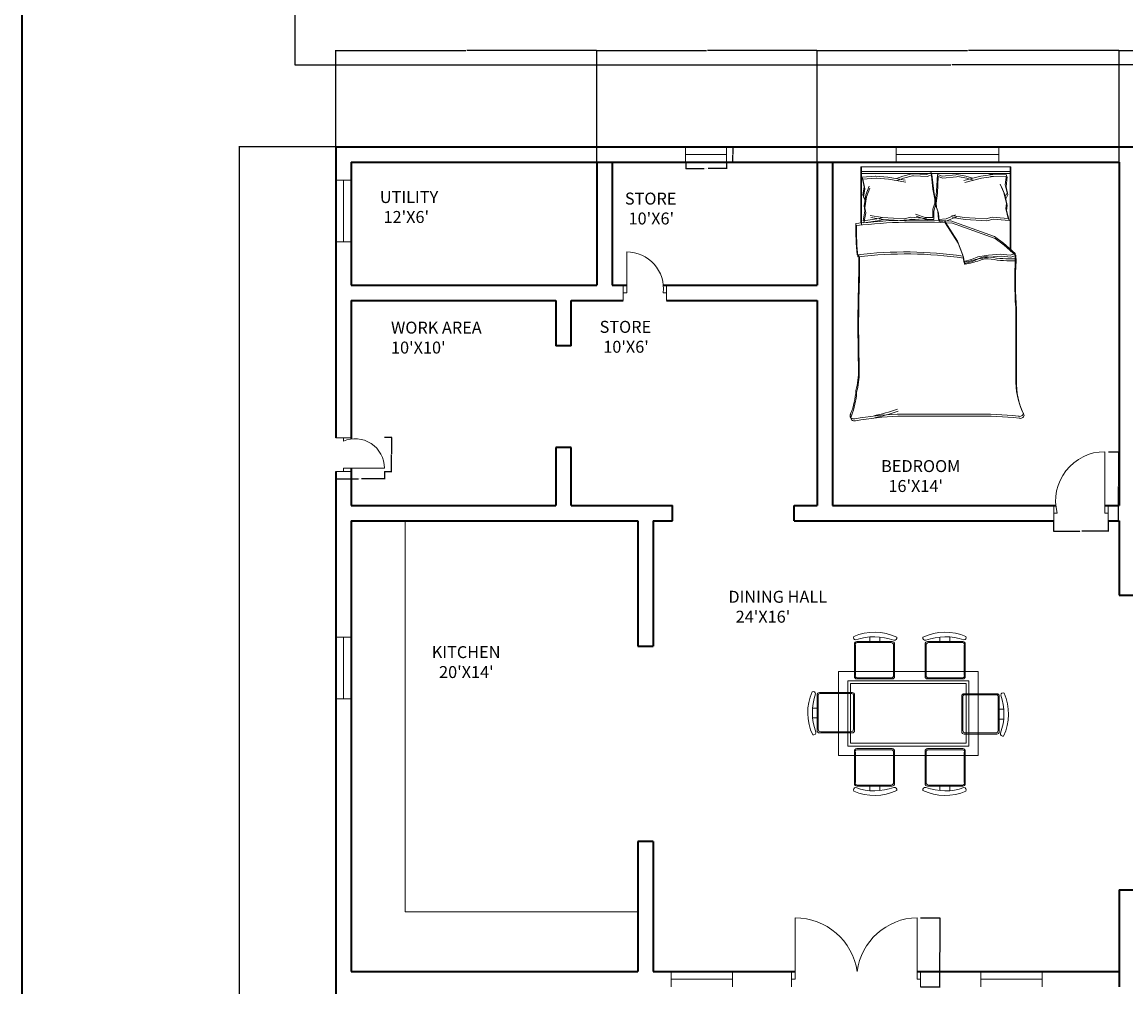
# Model space of a CAD drawing. Units: inches. Extents: x 2185 to 4426, y 1138 to 3073.
# Tile 5 of 14: x 2185 to 2832, y 1834 to 2400. Entities that reach past the tile are written whole.
import ezdxf

# ---------------------------------------------------------------- set-up
doc = ezdxf.new("R2010")
doc.units = ezdxf.units.IN
for name, color, linetype, lineweight in [('A-ANNO-DIMS', 2, 'Continuous', 18), ('A-ANNO-TTLB', 7, 'Continuous', 35), ('A-AREA-IDEN', 7, 'Continuous', 18), ('A-DOOR', 3, 'Continuous', 18), ('A-FLOR-CASE', 32, 'Continuous', 18), ('A-FURN', 8, 'Continuous', 18), ('A-GLAZ', 4, 'Continuous', 18), ('A-WALL', 7, 'Continuous', 35)]:
    doc.layers.add(name, color=color, linetype=linetype, lineweight=lineweight)
doc.styles.get("Standard").update_dxf_attribs({"font": 'arial.ttf'})
doc.dimstyles.get("Standard").update_dxf_attribs({"dimtxt": 0.18, "dimasz": 0.18, "dimexe": 0.18, "dimexo": 0.0625, "dimgap": 0.09, "dimtad": 0, "dimtih": 1, "dimtoh": 1, "dimdec": 4, "dimzin": 0, "dimdsep": 46, "dimtxsty": 'Standard', "dimcen": 0.09, "dimadec": 0, "dimazin": 0, "dimtfac": 1, "dimtdec": 4, "dimtofl": 0, "dimtmove": 0, "dimatfit": 3, "dimfxl": 1, "dimtolj": 1, "dimtzin": 0, "dimarcsym": 0})

# ---------------------------------------------------------------- blocks, each defined once
blk = doc.blocks.new('BED-DOUBLE')
for p, q in [((51.91, 97.09), (45.96, 90.32)), ((55.1, 97.24), (51.91, 97.09, 7.08)), ((53.04, 94.28), (51.91, 97.09)), ((0, 93.75), (0, 94.16)), ((0, 94.16), (1.36, 94.16)), ((0, 93.75), (48.66, 93.75)), ((0, 6.35), (0, 93.75)), ((1.17, 94.16), (49.83, 94.16)), ((2.8, 6.35), (2.8, 93.75)), ((3.97, 6.77), (3.97, 94.16)), ((4.68, 91.64), (4.5, 81.76)), ((4.68, 91.64), (10.55, 90.94)), ((5.85, 92.05), (5.67, 82.18)), ((5.85, 92.05), (11.72, 91.36)), ((10.55, 90.94), (15.25, 92.03)), ((16.27, 90.59), (11.37, 88.43)), ((11.72, 91.36), (16.42, 92.45)), ((21.63, 91.64), (15.1, 90.17)), ((15.25, 92.03), (17.16, 91.09)), ((22.8, 92.05), (16.27, 90.59)), ((16.42, 92.45), (18.33, 91.51)), ((24.57, 91.29), (21.63, 91.64)), ((25.74, 91.71), (22.8, 92.05)), ((30.31, 92.71), (24.57, 91.29)), ((31.48, 93.13), (25.74, 91.71)), ((29.57, 83.32), (30.31, 92.71)), ((30.74, 83.74), (31.48, 93.13)), ((50.74, 96.68), (44.79, 89.9)), ((53.93, 96.82), (50.74, 96.68, 7.08)), ((51.87, 93.87), (50.74, 96.68)), ((51.3, 88.2), (51.87, 93.87)), ((52.47, 88.62), (53.04, 94.28)), ((15.1, 90.17), (10.2, 88.01)), ((40.83, 84.52), (37.15, 74.32)), ((42, 84.94), (38.32, 74.74)), ((44.79, 89.9), (40.83, 84.52)), ((45.96, 90.32), (42, 84.94)), ((51.87, 81.12), (51.3, 88.2)), ((53.04, 81.54), (52.47, 88.62)), ((4.5, 81.76), (4.65, 83.59)), ((4.65, 83.59), (5.61, 76.65)), ((5.67, 82.18), (5.82, 84.01)), ((5.82, 84.01), (6.78, 77.06)), ((30.59, 79.74), (29.57, 83.32)), ((29.8, 66.92), (30.59, 79.74)), ((31.76, 80.16), (30.74, 83.74)), ((30.97, 67.34), (31.76, 80.16)), ((52.72, 74.89), (51.87, 81.12)), ((53.89, 75.31), (53.04, 81.54)), ((5.61, 76.65), (8.09, 66.74)), ((6.72, 71.68), (5.63, 67.91)), ((6.78, 77.06), (9.26, 67.15)), ((7.89, 72.1), (6.8, 68.32)), ((37.15, 74.32), (31.79, 59.08)), ((38.32, 74.74), (32.96, 59.49)), ((54.42, 71.21), (52.72, 74.89)), ((55.59, 71.63), (53.89, 75.31)), ((55.55, 66.68), (54.42, 71.21)), ((56.72, 67.09), (55.59, 71.63)), ((144.91, 27.55), (144.91, 72.56)), ((146.08, 27.96), (146.08, 72.97)), ((5.63, 67.91), (4.64, 62.55)), ((6.8, 68.32), (5.81, 62.97)), ((28.58, 59.55), (29.8, 66.92)), ((29.75, 59.97), (30.97, 67.34)), ((43.66, 63), (51.87, 66.11)), ((44.83, 63.41), (53.04, 66.53)), ((51.87, 66.11), (55.55, 66.68)), ((53.04, 66.53), (56.72, 67.09)), ((4.64, 62.55), (4.68, 61.96)), ((4.68, 61.96), (5.45, 53.86)), ((5.81, 62.97), (5.85, 62.38)), ((5.85, 62.38), (6.62, 54.28)), ((30.61, 56.23), (28.26, 61.85)), ((31.78, 56.65), (29.43, 62.26)), ((31.79, 55.33), (43.66, 63)), ((32.96, 55.75), (44.83, 63.41)), ((5.45, 53.86), (4.56, 51.16)), ((6.62, 54.28), (5.73, 51.58)), ((23.8, 50.59), (27.17, 51.86)), ((26, 51.44), (30.89, 51.75)), ((27.17, 51.86), (32.06, 52.16)), ((30.89, 51.75), (30.61, 56.23)), ((32.06, 52.16), (31.78, 56.65)), ((3.42, 47.51), (13.2, 48.57)), ((4.48, 44.87), (3.42, 47.51)), ((4.56, 51.16), (14.39, 50.71)), ((4.59, 47.93), (14.37, 48.99)), ((5.65, 45.29), (4.59, 47.93)), ((5.38, 37.16), (5.65, 45.29)), ((5.73, 51.58), (15.56, 51.13)), ((13.2, 48.57), (19.02, 49.63)), ((14.37, 48.99), (20.19, 50.05)), ((14.39, 50.71), (20.26, 50.02)), ((15.56, 51.13), (21.43, 50.44)), ((19.02, 49.63), (21.4, 49.63)), ((20.19, 50.05), (22.57, 50.05)), ((20.26, 50.02), (22.63, 50.17)), ((21.4, 49.63), (24.84, 48.57)), ((21.43, 50.44), (23.8, 50.59)), ((22.57, 50.05), (26.01, 48.99)), ((22.63, 50.17), (26, 51.44)), ((24.84, 48.57), (29.74, 48.57)), ((26.01, 48.99), (30.91, 48.99)), ((29.74, 48.57), (29.74, 44.08)), ((30.91, 48.99), (30.91, 44.49)), ((4.21, 36.74), (4.48, 44.87)), ((29.74, 44.08), (27.75, 38.33)), ((30.91, 44.49), (28.91, 38.74)), ((29.57, 35.45), (30.31, 44.83)), ((30.74, 35.86), (31.48, 45.25)), ((4.21, 36.15), (4.21, 36.74)), ((5.54, 30.86), (4.21, 36.15)), ((5.38, 36.57), (5.38, 37.16)), ((6.7, 31.28), (5.38, 36.57)), ((7.23, 22.56), (9.08, 32.6)), ((30.59, 31.86), (29.57, 35.45)), ((31.76, 32.28), (30.74, 35.86)), ((6.86, 27.16), (5.54, 30.86)), ((6.06, 22.14), (7.92, 32.19)), ((8.03, 27.58), (6.7, 31.28)), ((29.8, 19.04), (30.59, 31.86)), ((30.97, 19.46), (31.76, 32.28)), ((5.54, 15.15), (6.06, 22.14)), ((6.7, 15.57), (7.23, 22.56)), ((29.75, 12.09), (30.97, 19.46)), ((30.97, 19.46), (31.56, 17.39)), ((5.5, 14.96), (5.54, 15.15)), ((6.1, 7.13), (5.5, 14.96)), ((6.67, 15.37), (6.7, 15.57)), ((7.27, 7.55), (6.67, 15.37)), ((28.58, 11.67), (29.8, 19.04)), ((29.8, 19.04), (30.39, 16.97)), ((30.39, 16.97), (31.71, 7.65)), ((31.56, 17.39), (32.88, 8.07)), ((1.17, 6.77), (0, 6.77)), ((34.29, 6.77), (1.17, 6.77)), ((6.06, 7.12), (11.88, 8.18)), ((7.23, 7.54), (13.05, 8.6)), ((16.38, 9.24), (11.35, 11.09)), ((11.88, 8.18), (16.64, 7.39)), ((17.55, 9.65), (12.52, 11.5)), ((13.05, 8.6), (17.81, 7.8)), ((22.99, 8.18), (16.38, 9.24)), ((16.64, 7.39), (18.49, 8.44)), ((24.16, 8.6), (17.55, 9.65)), ((17.81, 7.8), (19.66, 8.86)), ((25.89, 8.71), (22.99, 8.18)), ((27.06, 9.13), (24.16, 8.6)), ((31.71, 7.65), (25.89, 8.71)), ((32.88, 8.07), (27.06, 9.13)), ((33.12, 6.35), (0, 6.35))]:
    blk.add_line(p, q)
for centre, radius, start, end in [((66.41, 333.3), 236.81, 266.97912, 273.83645), ((-11, 94.28), 66.17, 349.87628, 2.56571), ((67.58, 333.72), 236.81, 266.97912, 273.83645), ((124.02, -8244.93), 8342.06, 90.002168, 90.286887), ((125.19, -8244.52), 8342.06, 90.002168, 90.286887), ((125.57, 139.26), 42.18, 267.47136, 296.46809), ((126.74, 139.68), 42.18, 267.47136, 296.46809), ((144.23, 99.5), 2.02, 332.65876, 86.02002), ((388.18, 75.25), 243.28, 174.4998, 180.63509), ((145.4, 99.91), 2.02, 332.65876, 86.02002), ((389.35, 75.67), 243.28, 174.4998, 180.63509), ((-12.17, 93.86), 66.17, 349.87628, 2.56571), ((64.12, 79.99), 11.38, 168.6608, 203.73842), ((65.29, 80.41), 11.38, 168.6608, 203.73842), ((2.71, 56.97), 54.23, 10.66171, 19.88058), ((3.88, 57.39), 54.23, 10.66171, 19.88058), ((285.85, 32.47), 235.93, 171.78449, 186.90062), ((287.02, 32.89), 235.93, 171.78449, 186.90062), ((55.66, 66.99), 0.337, 250.24637, 1.13765), ((56.83, 67.41), 0.337, 250.24637, 1.13765), ((332.91, 39.06), 301.67, 176.08655, 186.78213), ((334.08, 39.47), 301.67, 176.08655, 186.78213), ((-43.36, -31.49), 194.68, 13.38322, 17.70533), ((-42.19, -31.08), 194.68, 13.38322, 17.70533), ((367.26, 39.18), 222.65, 182.99578, 189.40907), ((368.43, 39.6), 222.65, 182.99578, 189.40907), ((36.75, 155.73), 152.34, 268.72178, 275.60397), ((37.92, 156.15), 152.34, 268.72178, 275.60397), ((57.01, -305.95), 311.07, 88.4762, 91.00819), ((58.18, -305.53), 311.07, 88.4762, 91.00819), ((92.56, 886.57), 881.98, 268.22771, 271.71854), ((93.72, 886.99), 881.98, 268.22771, 271.71854), ((117.98, -49.19), 54.19, 76.06484, 88.91125), ((119.15, -48.77), 54.19, 76.06484, 88.91125), ((128.51, -39.61), 43.09, 67.97508, 86.652), ((129.68, -39.19), 43.09, 67.97508, 86.652), ((145.78, 1.99), 1.99, 236.17358, 23.47814), ((146.95, 2.41), 1.99, 236.17358, 23.47814)]:
    blk.add_arc(centre, radius, start, end)
blk = doc.blocks.new('DOOR-SGL-36-BED-W')
for p, q in [((29.94, 4.5), (29.94, 40.5)), ((0, 9), (0, 0)), ((31.94, 0), (31.94, 9)), ((31.94, 9), (31.94, 4.5)), ((0, 0), (0, 4.5)), ((0, 4.5), (2, 4.5)), ((31.94, 4.5), (29.94, 4.5)), ((0, 0), (0, 0))]:
    blk.add_line(p, q)
blk.add_arc((29.94, 11.66), 28.84, 90, 194.37957)
blk = doc.blocks.new('DOOR-SGL-24-STORE')
for p, q in [((2, 4.5), (2, 28.5)), ((0, 9), (0, 0)), ((25.41, 9), (25.41, 0)), ((0, 0), (0, 4.5)), ((0, 4.5), (2, 4.5)), ((25.41, 4.5), (23.41, 4.5)), ((25.41, 0), (25.41, 4.5))]:
    blk.add_line(p, q)
blk.add_arc((2, 6.95), 21.55, 353.47903, 90)
blk = doc.blocks.new('DOOR-SGL-24-WORK')
for p, q in [((9, 19.77), (0, 19.77)), ((0, 19.77), (4.5, 19.77)), ((4.5, 19.77), (4.5, 17.77)), ((9, 0), (0, 0)), ((0, 0), (4.5, 0)), ((4.5, 0), (4.5, 2)), ((4.5, 2), (28.5, 2))]:
    blk.add_line(p, q)
blk.add_arc((11.32, 2), 17.18, 0, 113.37775)
blk = doc.blocks.new('DOOR-PAIR-36-DINING')
for p, q in [((2, 4.5), (2, 40.5)), ((73.51, 4.5), (73.51, 40.5)), ((0, 9), (0, 0)), ((75.51, 0), (75.51, 9)), ((75.51, 9), (75.51, 4.5)), ((0, 0), (0, 4.5)), ((0, 4.5), (2, 4.5)), ((75.51, 4.5), (73.51, 4.5))]:
    blk.add_line(p, q)
for centre, radius, start, end in [((2, 3.7), 36.8, 8.27614, 90), ((74.14, 4.5), 36.01, 90.99344, 172.82033)]:
    blk.add_arc(centre, radius, start, end)
blk = doc.blocks.new('WIN-PLAN-24IN-01')
for p, q in [((0, 9), (0, 0)), ((24, 4.5), (24, 9)), ((24, 9), (24, 0)), ((0, 0), (0, 4.5)), ((0, 4.5), (0, 4.5)), ((0, 4.5), (24, 4.5))]:
    blk.add_line(p, q)
blk = doc.blocks.new('WIN-PLAN-36IN-01')
for p, q in [((0, 9), (0, 0)), ((36, 4.5), (36, 9)), ((36, 9), (36, 0)), ((0, 0), (0, 4.5)), ((0, 4.5), (0, 4.5)), ((0, 4.5), (36, 4.5))]:
    blk.add_line(p, q)
blk = doc.blocks.new('WIN-PLAN-36IN-02')
for p, q in [((9, 36), (0, 36)), ((0, 36), (4.5, 36)), ((4.5, 36), (4.5, 0)), ((9, 0), (0, 0)), ((4.5, 0), (9, 0))]:
    blk.add_line(p, q)
blk = doc.blocks.new('WIN-PLAN-60IN-02')
for p, q in [((0, 9), (0, 0)), ((60, 4.5), (60, 9)), ((60, 9), (60, 0)), ((0, 0), (0, 4.5)), ((0, 4.5), (0, 4.5)), ((0, 4.5), (60, 4.5)), ((0, 0), (0, 0))]:
    blk.add_line(p, q)
blk = doc.blocks.new('KITCHEN-COUNTER-L')
for p, q in [((0, 0), (0, 229.1)), ((136.38, 0), (0, 0)), ((136.38, 0), (136.38, 0))]:
    blk.add_line(p, q)
blk = doc.blocks.new('*D54')
at = {"layer": 'A-ANNO-DIMS', "color": 0, "lineweight": -2, "transparency": 16777216}
for p, q in [((2573.56, 2317.31), (2573.56, 2313.6)), ((2597.56, 2317.31), (2597.56, 2313.6)), ((2573.74, 2313.78), (2584.44, 2313.78)), ((2597.38, 2313.78), (2586.67, 2313.78))]:
    blk.add_line(p, q, dxfattribs=at)
at = {"layer": 'A-ANNO-DIMS', "color": 0, "transparency": 16777216}
for points in [[(2573.74, 2313.81), (2573.74, 2313.75), (2573.56, 2313.78)], [(2597.38, 2313.81), (2597.38, 2313.75), (2597.56, 2313.78)]]:
    blk.add_solid(points, dxfattribs=at)
at = {"layer": 'Defpoints', "color": 0, "transparency": 16777216}
for p in [(2573.56, 2317.38), (2597.56, 2317.38), (2597.56, 2313.78)]:
    blk.add_point(p, dxfattribs=at)
at = {"layer": 'A-ANNO-DIMS', "color": 0, "transparency": 16777216, "insert": (2585.56, 2313.78), "char_height": 0.18, "attachment_point": 5}
blk.add_mtext('\\A1;WINDOW 24 TYP.', dxfattribs=at)
blk = doc.blocks.new('*D55')
at = {"layer": 'A-ANNO-DIMS', "color": 0, "lineweight": -2, "transparency": 16777216}
for p, q in [((2597.62, 2326.38), (2601.34, 2326.38)), ((2601.16, 2326.2), (2601.16, 2322.06)), ((2597.62, 2317.38), (2601.34, 2317.38)), ((2601.16, 2317.56), (2601.16, 2321.7))]:
    blk.add_line(p, q, dxfattribs=at)
at = {"layer": 'A-ANNO-DIMS', "color": 0, "transparency": 16777216}
for points in [[(2601.13, 2326.2), (2601.19, 2326.2), (2601.16, 2326.38)], [(2601.13, 2317.56), (2601.19, 2317.56), (2601.16, 2317.38)]]:
    blk.add_solid(points, dxfattribs=at)
at = {"layer": 'Defpoints', "color": 0, "transparency": 16777216}
for p in [(2597.56, 2326.38), (2601.16, 2326.38), (2597.56, 2317.38)]:
    blk.add_point(p, dxfattribs=at)
at = {"layer": 'A-ANNO-DIMS', "color": 0, "transparency": 16777216, "insert": (2601.16, 2321.88), "char_height": 0.18, "attachment_point": 5}
blk.add_mtext('\\A1;9 TYP.', dxfattribs=at)
blk = doc.blocks.new('*D66')
at = {"layer": 'A-ANNO-DIMS', "color": 0, "lineweight": -2, "transparency": 16777216}
for p, q in [((2821.22, 2147.88), (2827.41, 2147.88)), ((2827.23, 2147.7), (2827.23, 2127.81)), ((2827.23, 2107.56), (2827.23, 2127.44)), ((2821.22, 2107.38), (2827.41, 2107.38))]:
    blk.add_line(p, q, dxfattribs=at)
at = {"layer": 'A-ANNO-DIMS', "color": 0, "transparency": 16777216}
for points in [[(2827.2, 2147.7), (2827.26, 2147.7), (2827.23, 2147.88)], [(2827.2, 2107.56), (2827.26, 2107.56), (2827.23, 2107.38)]]:
    blk.add_solid(points, dxfattribs=at)
at = {"layer": 'Defpoints', "color": 0, "transparency": 16777216}
for p in [(2821.16, 2147.88), (2827.23, 2147.88), (2821.16, 2107.38)]:
    blk.add_point(p, dxfattribs=at)
at = {"layer": 'A-ANNO-DIMS', "color": 0, "transparency": 16777216, "insert": (2827.23, 2127.63), "char_height": 0.18, "attachment_point": 5}
blk.add_mtext('\\A1;DOOR 41 TYP.', dxfattribs=at)
blk = doc.blocks.new('*D67')
at = {"layer": 'A-ANNO-DIMS', "color": 0, "lineweight": -2, "transparency": 16777216}
for p, q in [((2789.01, 2107.31), (2789.01, 2101.12)), ((2821.16, 2107.31), (2821.16, 2101.12)), ((2789.19, 2101.3), (2804.56, 2101.3)), ((2820.98, 2101.3), (2805.61, 2101.3))]:
    blk.add_line(p, q, dxfattribs=at)
at = {"layer": 'A-ANNO-DIMS', "color": 0, "transparency": 16777216}
for points in [[(2789.19, 2101.33), (2789.19, 2101.27), (2789.01, 2101.3)], [(2820.98, 2101.33), (2820.98, 2101.27), (2821.16, 2101.3)]]:
    blk.add_solid(points, dxfattribs=at)
at = {"layer": 'Defpoints', "color": 0, "transparency": 16777216}
for p in [(2789.01, 2107.38), (2821.16, 2107.38), (2821.16, 2101.3)]:
    blk.add_point(p, dxfattribs=at)
at = {"layer": 'A-ANNO-DIMS', "color": 0, "transparency": 16777216, "insert": (2805.08, 2101.3), "char_height": 0.18, "attachment_point": 5}
blk.add_mtext('\\A1;32 TYP.', dxfattribs=at)
blk = doc.blocks.new('*D70')
at = {"layer": 'A-ANNO-DIMS', "color": 0, "lineweight": -2, "transparency": 16777216}
for p, q in [((2368.52, 2136.24), (2368.52, 2131.85)), ((2397.02, 2136.24), (2397.02, 2131.85)), ((2368.7, 2132.03), (2381.83, 2132.03)), ((2396.84, 2132.03), (2383.71, 2132.03))]:
    blk.add_line(p, q, dxfattribs=at)
at = {"layer": 'A-ANNO-DIMS', "color": 0, "transparency": 16777216}
for points in [[(2368.7, 2132.06), (2368.7, 2132), (2368.52, 2132.03)], [(2396.84, 2132.06), (2396.84, 2132), (2397.02, 2132.03)]]:
    blk.add_solid(points, dxfattribs=at)
at = {"layer": 'Defpoints', "color": 0, "transparency": 16777216}
for p in [(2368.52, 2136.3), (2397.02, 2136.3), (2397.02, 2132.03)]:
    blk.add_point(p, dxfattribs=at)
at = {"layer": 'A-ANNO-DIMS', "color": 0, "transparency": 16777216, "insert": (2382.77, 2132.03), "char_height": 0.18, "attachment_point": 5}
blk.add_mtext('\\A1;DOOR 29 TYP.', dxfattribs=at)
blk = doc.blocks.new('*D71')
at = {"layer": 'A-ANNO-DIMS', "color": 0, "lineweight": -2, "transparency": 16777216}
for p, q in [((2397.08, 2156.37), (2401.47, 2156.37)), ((2401.29, 2156.19), (2401.29, 2146.52)), ((2401.29, 2136.48), (2401.29, 2146.15)), ((2397.08, 2136.3), (2401.47, 2136.3))]:
    blk.add_line(p, q, dxfattribs=at)
at = {"layer": 'A-ANNO-DIMS', "color": 0, "transparency": 16777216}
for points in [[(2401.26, 2156.19), (2401.32, 2156.19), (2401.29, 2156.37)], [(2401.26, 2136.48), (2401.32, 2136.48), (2401.29, 2136.3)]]:
    blk.add_solid(points, dxfattribs=at)
at = {"layer": 'Defpoints', "color": 0, "transparency": 16777216}
for p in [(2397.02, 2156.37), (2401.29, 2156.37), (2397.02, 2136.3)]:
    blk.add_point(p, dxfattribs=at)
at = {"layer": 'A-ANNO-DIMS', "color": 0, "transparency": 16777216, "insert": (2401.29, 2146.34), "char_height": 0.18, "attachment_point": 5}
blk.add_mtext('\\A1;20 TYP.', dxfattribs=at)
blk = doc.blocks.new('*D77')
at = {"layer": 'A-ANNO-DIMS', "color": 0, "lineweight": -2, "transparency": 16777216}
for p, q in [((2711.22, 1874.88), (2722.66, 1874.88)), ((2722.48, 1874.7), (2722.48, 1854.81)), ((2722.48, 1834.56), (2722.48, 1854.45)), ((2711.22, 1834.38), (2722.66, 1834.38))]:
    blk.add_line(p, q, dxfattribs=at)
at = {"layer": 'A-ANNO-DIMS', "color": 0, "transparency": 16777216}
for points in [[(2722.45, 1874.7), (2722.51, 1874.7), (2722.48, 1874.88)], [(2722.45, 1834.56), (2722.51, 1834.56), (2722.48, 1834.38)]]:
    blk.add_solid(points, dxfattribs=at)
at = {"layer": 'Defpoints', "color": 0, "transparency": 16777216}
for p in [(2711.16, 1874.88), (2722.48, 1874.88), (2711.16, 1834.38)]:
    blk.add_point(p, dxfattribs=at)
at = {"layer": 'A-ANNO-DIMS', "color": 0, "transparency": 16777216, "insert": (2722.48, 1854.63), "char_height": 0.18, "attachment_point": 5}
blk.add_mtext('\\A1;41 TYP.', dxfattribs=at)
blk = doc.blocks.new('*D139')
at = {"layer": 'A-ANNO-DIMS', "color": 0, "lineweight": -2, "transparency": 16777216}
for p, q in [((2368.46, 2326.38), (2311.84, 2326.38)), ((2312.02, 2326.2), (2312.02, 1827.06)), ((2312.02, 1327.56), (2312.02, 1826.7)), ((2368.46, 1327.38), (2311.84, 1327.38))]:
    blk.add_line(p, q, dxfattribs=at)
at = {"layer": 'A-ANNO-DIMS', "color": 0, "transparency": 16777216}
for points in [[(2311.99, 2326.2), (2312.05, 2326.2), (2312.02, 2326.38)], [(2311.99, 1327.56), (2312.05, 1327.56), (2312.02, 1327.38)]]:
    blk.add_solid(points, dxfattribs=at)
at = {"layer": 'Defpoints', "color": 0, "transparency": 16777216}
for p in [(2312.02, 2326.38), (2368.52, 2326.38), (2368.52, 1327.38)]:
    blk.add_point(p, dxfattribs=at)
at = {"layer": 'A-ANNO-DIMS', "color": 0, "transparency": 16777216, "insert": (2312.02, 1826.88), "char_height": 0.18, "attachment_point": 5}
blk.add_mtext('\\A1;999', dxfattribs=at)
blk = doc.blocks.new('*D140')
at = {"layer": 'A-ANNO-DIMS', "color": 0, "lineweight": -2, "transparency": 16777216}
for p, q in [((2368.52, 2326.44), (2368.52, 2383.06)), ((2368.7, 2382.88), (2444.74, 2382.88)), ((2521.34, 2382.88), (2445.3, 2382.88)), ((2521.52, 2317.44), (2521.52, 2383.06))]:
    blk.add_line(p, q, dxfattribs=at)
at = {"layer": 'A-ANNO-DIMS', "color": 0, "transparency": 16777216}
for points in [[(2368.7, 2382.91), (2368.7, 2382.85), (2368.52, 2382.88)], [(2521.34, 2382.91), (2521.34, 2382.85), (2521.52, 2382.88)]]:
    blk.add_solid(points, dxfattribs=at)
at = {"layer": 'Defpoints', "color": 0, "transparency": 16777216}
for p in [(2521.52, 2382.88), (2368.52, 2326.38), (2521.52, 2317.38)]:
    blk.add_point(p, dxfattribs=at)
at = {"layer": 'A-ANNO-DIMS', "color": 0, "transparency": 16777216, "insert": (2445.02, 2382.88), "char_height": 0.18, "attachment_point": 5}
blk.add_mtext('\\A1;153', dxfattribs=at)
blk = doc.blocks.new('*D141')
at = {"layer": 'A-ANNO-DIMS', "color": 0, "lineweight": -2, "transparency": 16777216}
for p, q in [((2521.52, 2317.44), (2521.52, 2383.06)), ((2521.7, 2382.88), (2585.74, 2382.88)), ((2650.34, 2382.88), (2586.3, 2382.88)), ((2650.52, 2317.44), (2650.52, 2383.06))]:
    blk.add_line(p, q, dxfattribs=at)
at = {"layer": 'A-ANNO-DIMS', "color": 0, "transparency": 16777216}
for points in [[(2521.7, 2382.91), (2521.7, 2382.85), (2521.52, 2382.88)], [(2650.34, 2382.91), (2650.34, 2382.85), (2650.52, 2382.88)]]:
    blk.add_solid(points, dxfattribs=at)
at = {"layer": 'Defpoints', "color": 0, "transparency": 16777216}
for p in [(2650.52, 2382.88), (2521.52, 2317.38), (2650.52, 2317.38)]:
    blk.add_point(p, dxfattribs=at)
at = {"layer": 'A-ANNO-DIMS', "color": 0, "transparency": 16777216, "insert": (2586.02, 2382.88), "char_height": 0.18, "attachment_point": 5}
blk.add_mtext('\\A1;129', dxfattribs=at)
blk = doc.blocks.new('*D142')
at = {"layer": 'A-ANNO-DIMS', "color": 0, "lineweight": -2, "transparency": 16777216}
for p, q in [((2650.52, 2317.44), (2650.52, 2383.06)), ((2650.7, 2382.88), (2738.74, 2382.88)), ((2827.34, 2382.88), (2739.3, 2382.88)), ((2827.52, 2317.44), (2827.52, 2383.06))]:
    blk.add_line(p, q, dxfattribs=at)
at = {"layer": 'A-ANNO-DIMS', "color": 0, "transparency": 16777216}
for points in [[(2650.7, 2382.91), (2650.7, 2382.85), (2650.52, 2382.88)], [(2827.34, 2382.91), (2827.34, 2382.85), (2827.52, 2382.88)]]:
    blk.add_solid(points, dxfattribs=at)
at = {"layer": 'Defpoints', "color": 0, "transparency": 16777216}
for p in [(2827.52, 2382.88), (2650.52, 2317.38), (2827.52, 2317.38)]:
    blk.add_point(p, dxfattribs=at)
at = {"layer": 'A-ANNO-DIMS', "color": 0, "transparency": 16777216, "insert": (2739.02, 2382.88), "char_height": 0.18, "attachment_point": 5}
blk.add_mtext('\\A1;177', dxfattribs=at)
blk = doc.blocks.new('*D143')
at = {"layer": 'A-ANNO-DIMS', "color": 0, "lineweight": -2, "transparency": 16777216}
for p, q in [((2827.52, 2317.44), (2827.52, 2383.06)), ((2827.7, 2382.88), (2867.82, 2382.88)), ((2908.34, 2382.88), (2868.22, 2382.88)), ((2908.52, 2317.44), (2908.52, 2383.06))]:
    blk.add_line(p, q, dxfattribs=at)
at = {"layer": 'A-ANNO-DIMS', "color": 0, "transparency": 16777216}
for points in [[(2827.7, 2382.91), (2827.7, 2382.85), (2827.52, 2382.88)], [(2908.34, 2382.91), (2908.34, 2382.85), (2908.52, 2382.88)]]:
    blk.add_solid(points, dxfattribs=at)
at = {"layer": 'Defpoints', "color": 0, "transparency": 16777216}
for p in [(2908.52, 2382.88), (2827.52, 2317.38), (2908.52, 2317.38)]:
    blk.add_point(p, dxfattribs=at)
at = {"layer": 'A-ANNO-DIMS', "color": 0, "transparency": 16777216, "insert": (2868.02, 2382.88), "char_height": 0.18, "attachment_point": 5}
blk.add_mtext('\\A1;81', dxfattribs=at)
blk = doc.blocks.new('*D162')
at = {"layer": 'A-ANNO-DIMS', "color": 0, "lineweight": -2, "transparency": 16777216}
for p, q in [((2344.52, 2611.42), (2344.52, 2374.27)), ((3114.02, 2611.42), (3114.02, 2374.27)), ((2344.7, 2374.45), (2728.88, 2374.45)), ((3113.84, 2374.45), (2729.66, 2374.45))]:
    blk.add_line(p, q, dxfattribs=at)
at = {"layer": 'A-ANNO-DIMS', "color": 0, "transparency": 16777216}
for points in [[(2344.7, 2374.48), (2344.7, 2374.42), (2344.52, 2374.45)], [(3113.84, 2374.48), (3113.84, 2374.42), (3114.02, 2374.45)]]:
    blk.add_solid(points, dxfattribs=at)
at = {"layer": 'Defpoints', "color": 0, "transparency": 16777216}
for p in [(2344.52, 2611.48), (3114.02, 2611.48), (3114.02, 2374.45)]:
    blk.add_point(p, dxfattribs=at)
at = {"layer": 'A-ANNO-DIMS', "color": 0, "transparency": 16777216, "insert": (2729.27, 2374.45), "char_height": 0.18, "attachment_point": 5}
blk.add_mtext('\\A1;769.5', dxfattribs=at)

msp = doc.modelspace()

# ---------------------------------------------------------------- linework, layer by layer
at = {"layer": 'A-ANNO-TTLB'}
msp.add_lwpolyline([(2184.741, 3073.364), (4426.252, 3073.364), (4426.252, 1137.99), (2184.741, 1137.99)], close=True, dxfattribs=at)
at = {"layer": 'A-FURN'}
for points in [[(2673.188, 2037.582, -0.1758092), (2695.509, 2037.413, 0.5783921), (2697.2, 2039.272, 0.2145244), (2672.004, 2039.61, 0.552014), (2673.188, 2037.582, -0.065079)], [(2687.283, 2036.686), (2687.283, 2039.307, -0.0647586)], [(2714.301, 2037.413, -0.5783921), (2712.61, 2039.272, -0.2145244), (2737.805, 2039.61, -0.552014), (2736.622, 2037.582, 0.1758092), (2714.301, 2037.413)], [(2722.526, 2036.686), (2722.526, 2039.307, 0.0647586)], [(2694.562, 2036.686), (2673.84, 2036.686, 0.4142136), (2672.39, 2035.236), (2672.39, 2016.183, 0.4142136), (2673.84, 2014.733), (2694.562, 2014.733, 0.4142136), (2696.012, 2016.183), (2696.012, 2035.236, 0.4142136), (2694.562, 2036.686)], [(2735.97, 2036.686, -0.4142136), (2737.419, 2035.236), (2737.419, 2016.183, -0.4142136), (2735.97, 2014.733), (2715.248, 2014.733, -0.4142136), (2713.798, 2016.183), (2713.798, 2035.236, -0.4142136), (2715.248, 2036.686), (2735.97, 2036.686)], [(2649.836, 1983.68, -0.5783921), (2647.977, 1981.989, -0.2145244), (2647.638, 2007.185, -0.552014), (2649.667, 2006.001, 0.1758094), (2649.836, 1983.68)], [(2650.563, 2005.349, -0.4142136), (2652.012, 2006.799), (2671.066, 2006.799, -0.4142136), (2672.516, 2005.349), (2672.516, 1984.627, -0.4142136), (2671.066, 1983.177), (2652.012, 1983.177, -0.4142136), (2650.563, 1984.627), (2650.563, 2005.349)], [(2757.272, 2004.639, 0.4142136), (2755.822, 2006.089), (2736.769, 2006.089, 0.4142136), (2735.319, 2004.639), (2735.319, 1983.917, 0.4142136), (2736.769, 1982.468), (2755.822, 1982.468, 0.4142136), (2757.272, 1983.917), (2757.272, 2004.639)], [(2758.168, 2005.291, -0.1758092), (2757.999, 1982.97, 0.5783921), (2759.858, 1981.279, 0.2145244), (2760.196, 2006.475, 0.552014), (2758.168, 2005.291, -0.065079)], [(2650.563, 1991.906), (2647.942, 1991.906, 0.0647586)], [(2757.272, 1991.196), (2759.893, 1991.196, -0.0647586)], [(2694.562, 1951.988), (2673.84, 1951.988, -0.4142136), (2672.39, 1953.438), (2672.39, 1972.492, -0.4142136), (2673.84, 1973.941), (2694.562, 1973.941, -0.4142136), (2696.012, 1972.492), (2696.012, 1953.438, -0.4142136), (2694.562, 1951.988)], [(2735.97, 1951.988, 0.4142136), (2737.419, 1953.438), (2737.419, 1972.492, 0.4142136), (2735.97, 1973.941), (2715.248, 1973.941, 0.4142136), (2713.798, 1972.492), (2713.798, 1953.438, 0.4142136), (2715.248, 1951.988), (2735.97, 1951.988)], [(2695.509, 1951.261, -0.5783921), (2697.2, 1949.402, -0.2145244), (2672.004, 1949.064, -0.552014), (2673.188, 1951.092, 0.1758093), (2695.509, 1951.261)], [(2687.283, 1951.988), (2687.283, 1949.367, 0.0647586)], [(2736.622, 1951.092, -0.1758093), (2714.301, 1951.261, 0.5783921), (2712.61, 1949.402, 0.2145244), (2737.805, 1949.064, 0.552014), (2736.622, 1951.092, -0.065079)], [(2722.526, 1951.988), (2722.526, 1949.367, -0.0647586)]]:
    msp.add_lwpolyline(points, format="xyb", dxfattribs=at)
for points in [[(2681.483, 2039.354), (2681.483, 2036.686)], [(2728.327, 2039.354), (2728.327, 2036.686)], [(2647.894, 1997.706), (2650.563, 1997.706)], [(2759.94, 1996.996), (2757.272, 1996.996)], [(2681.483, 1949.32), (2681.483, 1951.988)], [(2728.327, 1949.32), (2728.327, 1951.988)]]:
    msp.add_lwpolyline(points, dxfattribs=at)
for points in [[(2673.849, 2036.033), (2693.909, 2036.033, -0.4142136), (2695.359, 2034.583), (2695.359, 2016.836, -0.4142136), (2693.909, 2015.386), (2673.849, 2015.386, -0.5120695), (2673.043, 2016.836), (2673.043, 2034.583, -0.5120695)], [(2735.961, 2036.033), (2715.901, 2036.033, 0.4142136), (2714.451, 2034.583), (2714.451, 2016.836, 0.4142136), (2715.901, 2015.386), (2735.961, 2015.386, 0.5120695), (2736.766, 2016.836), (2736.766, 2034.583, 0.5120695)], [(2651.216, 2005.34), (2651.216, 1985.28, 0.4142136), (2652.666, 1983.83), (2670.413, 1983.83, 0.4142136), (2671.863, 1985.28), (2671.863, 2005.34, 0.5120695), (2670.413, 2006.146), (2652.666, 2006.146, 0.5120695)], [(2756.619, 2004.631), (2756.619, 1984.57, -0.4142136), (2755.169, 1983.121), (2737.422, 1983.121, -0.4142136), (2735.972, 1984.57), (2735.972, 2004.631, -0.5120695), (2737.422, 2005.436), (2755.169, 2005.436, -0.5120695)], [(2673.849, 1952.641), (2693.909, 1952.641, 0.4142136), (2695.359, 1954.091), (2695.359, 1971.838, 0.4142136), (2693.909, 1973.288), (2673.849, 1973.288, 0.5120695), (2673.043, 1971.838), (2673.043, 1954.091, 0.5120695)], [(2735.961, 1952.641), (2715.901, 1952.641, -0.4142136), (2714.451, 1954.091), (2714.451, 1971.838, -0.4142136), (2715.901, 1973.288), (2735.961, 1973.288, -0.5120695), (2736.766, 1971.838), (2736.766, 1954.091, -0.5120695)]]:
    msp.add_lwpolyline(points, format="xyb", close=True, dxfattribs=at)
for points in [[(2663.052, 2019.186), (2745.002, 2019.186), (2745.002, 1970.015), (2663.052, 1970.015)], [(2668.515, 2013.722), (2739.539, 2013.722), (2739.539, 1975.479), (2668.515, 1975.479)], [(2670.154, 2012.083), (2737.9, 2012.083), (2737.9, 1977.118), (2670.154, 1977.118)]]:
    msp.add_lwpolyline(points, close=True, dxfattribs=at)
at = {"layer": 'A-WALL'}
for p, q in [((2368.519, 2326.377), (2368.519, 2156.075)), ((2368.519, 2326.377), (2368.519, 2156.075)), ((2368.519, 2326.377), (3090.019, 2326.377)), ((2377.519, 2317.377), (2827.519, 2317.377)), ((2377.519, 2317.377), (2377.519, 2245.377)), ((2521.519, 2317.377), (2521.519, 2245.377)), ((2530.519, 2317.377), (2530.519, 2245.377)), ((2650.519, 2317.377), (2650.519, 2245.377)), ((2659.519, 2317.377), (2659.519, 2116.377)), ((2827.519, 2317.377), (2827.519, 2116.377)), ((2377.519, 2245.377), (2521.519, 2245.377)), ((2530.519, 2245.377), (2538.99, 2245.377)), ((2560.445, 2245.377), (2650.519, 2245.377)), ((2377.519, 2236.377), (2497.519, 2236.377)), ((2377.519, 2236.377), (2377.519, 2155.328)), ((2377.519, 2236.377), (2497.519, 2236.377)), ((2497.519, 2236.377), (2497.519, 2209.971)), ((2506.519, 2236.377), (2530.519, 2236.377)), ((2506.519, 2209.971), (2506.519, 2236.377)), ((2530.519, 2236.377), (2536.99, 2236.377)), ((2562.403, 2236.377), (2650.519, 2236.377)), ((2650.519, 2236.377), (2650.519, 2116.377)), ((2506.519, 2209.971), (2497.519, 2209.971)), ((2506.519, 2150.249), (2497.519, 2150.249)), ((2497.519, 2150.249), (2497.519, 2116.377)), ((2506.519, 2116.377), (2506.519, 2150.249)), ((2368.519, 2136.303), (2368.519, 1327.377)), ((2368.519, 2136.303), (2368.519, 1327.377)), ((2377.519, 2138.303), (2377.519, 2116.377)), ((2377.519, 2116.377), (2497.519, 2116.377)), ((2506.519, 2116.377), (2530.519, 2116.377)), ((2530.519, 2116.377), (2565.808, 2116.377)), ((2565.808, 2107.377), (2565.808, 2116.377)), ((2637.085, 2107.377), (2637.085, 2116.377)), ((2637.085, 2116.377), (2650.519, 2116.377)), ((2659.519, 2116.377), (2790.443, 2116.377)), ((2819.158, 2116.377), (2827.519, 2116.377)), ((2377.519, 2107.377), (2521.519, 2107.377)), ((2377.519, 2107.377), (2377.519, 1843.377)), ((2521.519, 2107.377), (2545.519, 2107.377)), ((2545.519, 2107.377), (2545.519, 2033.934)), ((2554.519, 2107.377), (2554.519, 2033.934)), ((2554.519, 2107.377), (2565.808, 2107.377)), ((2637.085, 2107.377), (2789.223, 2107.377)), ((2821.158, 2107.377), (2827.519, 2107.377)), ((2827.519, 2107.377), (2827.519, 2063.852)), ((2827.519, 2063.852), (2836.519, 2063.852)), ((2545.519, 2033.934), (2554.519, 2033.934)), ((2554.519, 1919.604), (2545.519, 1919.604)), ((2545.519, 1919.604), (2545.519, 1843.377)), ((2554.519, 1919.604), (2554.519, 1843.377)), ((2377.519, 1906.377), (2377.519, 1843.377)), ((2827.519, 1891.155), (2836.519, 1891.155)), ((2827.519, 1891.155), (2827.519, 1843.377)), ((2377.519, 1843.377), (2521.519, 1843.377)), ((2521.519, 1843.377), (2545.519, 1843.377)), ((2554.519, 1843.377), (2637.644, 1843.377)), ((2709.156, 1843.377), (2827.519, 1843.377)), ((2827.519, 1843.377), (2827.519, 1834.377))]:
    msp.add_line(p, q, dxfattribs=at)

# ---------------------------------------------------------------- block references
at = {"layer": 'A-DOOR'}
for name, p in [('DOOR-SGL-24-STORE', (2536.99, 2236.377)), ('DOOR-SGL-24-WORK', (2368.519, 2136.303)), ('DOOR-SGL-36-BED-W', (2789.223, 2107.377)), ('DOOR-PAIR-36-DINING', (2635.644, 1834.377))]:
    msp.add_blockref(name, p, dxfattribs=at)
at = {"layer": 'A-FLOR-CASE'}
msp.add_blockref('KITCHEN-COUNTER-L', (2409.143, 1878.273), dxfattribs=at)
at = {"layer": 'A-FURN', "rotation": 270.0000000000001}
msp.add_blockref('BED-DOUBLE', (2669.901, 2314.794), dxfattribs=at)
at = {"layer": 'A-GLAZ'}
for name, p in [('WIN-PLAN-24IN-01', (2573.556, 2317.377)), ('WIN-PLAN-60IN-02', (2696.982, 2317.377)), ('WIN-PLAN-36IN-02', (2368.519, 2270.862)), ('WIN-PLAN-36IN-01', (2746.431, 1834.377))]:
    msp.add_blockref(name, p, dxfattribs=at)
for name, p, rotation in [('WIN-PLAN-36IN-01', (2368.519, 2039.2), 270.0000000000013), ('WIN-PLAN-36IN-02', (2601.039, 1834.377), 90.00000000000102)]:
    msp.add_blockref(name, p, dxfattribs=dict(at, rotation=rotation))

# ---------------------------------------------------------------- texts
at = {"layer": 'A-AREA-IDEN', "char_height": 7, "attachment_point": 1}
for s, width, insert in [("UTILITY\\P 12'X6'", 95.53712, (2394.38, 2300.521)), ("STORE\\P 10'X6'", 76.14613, (2537.955, 2299.622)), ("STORE\\P 10'X6'", 117.12364, (2523.141, 2224.486)), ("BEDROOM\\P  16'X14'", 127.66196, (2688.078, 2142.94)), ("DINING HALL\\P  24'X16'", 193.6148, (2598.582, 2066.382)), ("KITCHEN\\P  20'X14'", 114.45156, (2424.798, 2033.983))]:
    msp.add_mtext_dynamic_manual_height_columns(s, width=width, gutter_width=12.5, heights=[0], dxfattribs=dict(at, insert=insert))
at = {"layer": 'A-AREA-IDEN', "insert": (2400.912, 2224.037), "char_height": 7, "width": 79.21159, "attachment_point": 1}
msp.add_mtext("WORK AREA\\P   10'X10'", dxfattribs=at)

# ---------------------------------------------------------------- dimensions: what is measured, and where the dimension line sits
at = {"layer": 'A-ANNO-DIMS'}
for base, p1, p2, override, picture, middle in [((3114.019, 2374.451), (2344.519, 2611.482), (3114.019, 2611.482), {"dimdec": 1, "dimlfac": 1, "dimrnd": 0, "dimzin": 0, "dimdsep": 46, "dimlunit": 2}, '*D162', (2729.269, 2374.451)), ((2521.519, 2382.877), (2368.519, 2326.377), (2521.519, 2317.377), {"dimdec": 0, "dimlfac": 1, "dimrnd": 0, "dimzin": 0, "dimdsep": 46, "dimlunit": 2}, '*D140', (2445.019, 2382.877)), ((2650.519, 2382.877), (2521.519, 2317.377), (2650.519, 2317.377), {"dimdec": 0, "dimlfac": 1, "dimrnd": 0, "dimzin": 0, "dimdsep": 46, "dimlunit": 2}, '*D141', (2586.019, 2382.877)), ((2827.519, 2382.877), (2650.519, 2317.377), (2827.519, 2317.377), {"dimdec": 0, "dimlfac": 1, "dimrnd": 0, "dimzin": 0, "dimdsep": 46, "dimlunit": 2}, '*D142', (2739.019, 2382.877)), ((2908.519, 2382.877), (2827.519, 2317.377), (2908.519, 2317.377), {"dimdec": 0, "dimlfac": 1, "dimrnd": 0, "dimzin": 0, "dimdsep": 46, "dimlunit": 2}, '*D143', (2868.019, 2382.877))]:
    dim = msp.add_linear_dim(base=base, p1=p1, p2=p2, dimstyle='Standard', override=override, dxfattribs=at)
    dim.commit()
    dim.dimension.update_dxf_attribs({"geometry": picture, "text_midpoint": middle})
dim = msp.add_linear_dim(base=(2312.019, 2326.377), p1=(2368.519, 1327.377), p2=(2368.519, 2326.377), angle=90, dimstyle='Standard', override={"dimdec": 0, "dimlfac": 1, "dimrnd": 0, "dimzin": 0, "dimdsep": 46, "dimlunit": 2}, dxfattribs=at)
dim.commit()
dim.dimension.update_dxf_attribs({"geometry": '*D139', "text_midpoint": (2312.019, 1826.877)})
for base, p1, p2, text, picture, middle in [((2601.156, 2326.377), (2597.556, 2317.377), (2597.556, 2326.377), '<> TYP.', '*D55', (2601.156, 2321.877)), ((2401.294, 2156.37), (2397.019, 2136.303), (2397.019, 2156.37), '<> TYP.', '*D71', (2401.294, 2146.337)), ((2827.233218203, 2147.876947079), (2821.158218203, 2107.376947079), (2821.158218203, 2147.876947079), 'DOOR <> TYP.', '*D66', (2827.233218203, 2127.626947079)), ((2722.483242552, 1874.876947079), (2711.156398771, 1834.376947079), (2711.156398771, 1874.876947079), '<> TYP.', '*D77', (2722.483242552, 1854.626947079))]:
    dim = msp.add_linear_dim(base=base, p1=p1, p2=p2, angle=90, text=text, dimstyle='Standard', override={"dimdec": 0, "dimlfac": 1, "dimrnd": 0, "dimzin": 0, "dimdsep": 46, "dimlunit": 2}, dxfattribs=at)
    dim.commit()
    dim.dimension.update_dxf_attribs({"geometry": picture, "text_midpoint": middle})
for base, p1, p2, text, picture, middle in [((2597.556, 2313.777), (2573.556, 2317.377), (2597.556, 2317.377), 'WINDOW <> TYP.', '*D54', (2585.556, 2313.777)), ((2397.019297542, 2132.028169998), (2368.519297542, 2136.303169998), (2397.019297542, 2136.303169998), 'DOOR <> TYP.', '*D70', (2382.769297542, 2132.028169998)), ((2821.158, 2101.302), (2789.011, 2107.377), (2821.158, 2107.377), '<> TYP.', '*D67', (2805.084, 2101.302))]:
    dim = msp.add_linear_dim(base=base, p1=p1, p2=p2, text=text, dimstyle='Standard', override={"dimdec": 0, "dimlfac": 1, "dimrnd": 0, "dimzin": 0, "dimdsep": 46, "dimlunit": 2}, dxfattribs=at)
    dim.commit()
    dim.dimension.update_dxf_attribs({"geometry": picture, "text_midpoint": middle})

doc.saveas('drawing.dxf')
